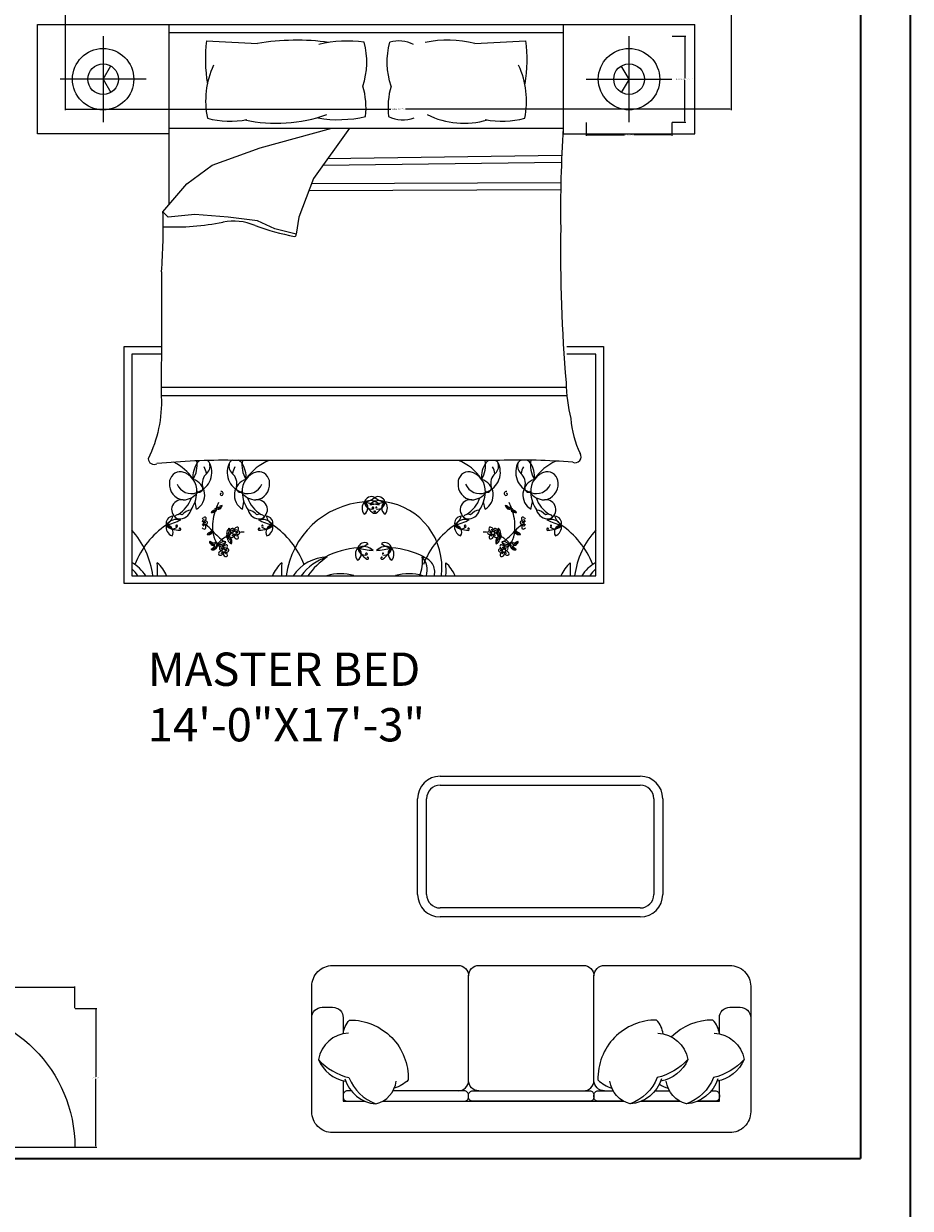
# Model space of a CAD drawing. Units: inches. Extents: x -10 to 502, y -868 to 56.
# Tile 13 of 14: x 298 to 458, y -264 to -50. Entities that reach past the tile are written whole.
import ezdxf

# ---------------------------------------------------------------- set-up
doc = ezdxf.new("R2010")
doc.units = ezdxf.units.IN
doc.header["$MEASUREMENT"] = 0
for name, color, linetype, lineweight in [('A-ANNO-DIMS', 2, 'Continuous', 18), ('A-AREA-IDEN', 7, 'Continuous', 18), ('A-DOOR', 4, 'Continuous', 25), ('A-FURN', 8, 'Continuous', 13), ('A-WALL', 7, 'Continuous', 35)]:
    doc.layers.add(name, color=color, linetype=linetype, lineweight=lineweight)
doc.styles.get("Standard").update_dxf_attribs({"font": 'arial.ttf'})
doc.dimstyles.get("Standard").update_dxf_attribs({"dimtxt": 0.18, "dimasz": 0.18, "dimexe": 0.18, "dimexo": 0.0625, "dimgap": 0.09, "dimtad": 0, "dimtih": 1, "dimtoh": 1, "dimdec": 0, "dimzin": 0, "dimdsep": 46, "dimlunit": 3, "dimtxsty": 'Standard', "dimcen": 0.09, "dimadec": 0, "dimazin": 0, "dimtfac": 1, "dimtdec": 0, "dimtofl": 0, "dimtmove": 0, "dimatfit": 3, "dimfxl": 1, "dimtolj": 1, "dimtzin": 0, "dimarcsym": 0})

# ---------------------------------------------------------------- blocks, each defined once
blk = doc.blocks.new('DOOR-SWING-25IN')
blk.add_line((25, 0), (0, 0))
blk.add_arc((25, 0), 25, 90, 180)
blk = doc.blocks.new('LAMP-BEDSIDE-LARGE')
for p, q in [((7.74, 0), (7.74, 15.47)), ((0, 7.74), (15.47, 7.74))]:
    blk.add_line(p, q)
for points in [[(7.74, 7.74), (6.35, 10.13)], [(7.74, 7.74), (6.35, 5.34)]]:
    blk.add_lwpolyline(points)
for radius in [5.53, 2.76]:
    blk.add_circle((7.74, 7.74), radius)
blk = doc.blocks.new('*D21')
at = {"layer": 'A-ANNO-DIMS', "color": 0, "lineweight": -2, "transparency": 16777216}
for p, q in [((305.7, -47.92), (305.7, -66.03)), ((425.7, -47.92), (425.7, -66.03)), ((305.88, -65.85), (364.4, -65.85)), ((425.52, -65.85), (367, -65.85))]:
    blk.add_line(p, q, dxfattribs=at)
at = {"layer": 'A-ANNO-DIMS', "color": 0, "transparency": 16777216}
for points in [[(305.88, -65.82), (305.88, -65.88), (305.7, -65.85)], [(425.52, -65.82), (425.52, -65.88), (425.7, -65.85)]]:
    blk.add_solid(points, dxfattribs=at)
at = {"layer": 'Defpoints', "color": 0, "transparency": 16777216}
for p in [(305.7, -47.85), (425.7, -47.85), (425.7, -65.85)]:
    blk.add_point(p, dxfattribs=at)
at = {"layer": 'A-ANNO-DIMS', "color": 0, "transparency": 16777216, "insert": (365.7, -65.85), "char_height": 0.18, "attachment_point": 5}
blk.add_mtext('\\A1;WINDOW 10\'-0" TYP.', dxfattribs=at)
blk = doc.blocks.new('*D25')
at = {"layer": 'A-ANNO-DIMS', "color": 0, "lineweight": -2, "transparency": 16777216}
for p, q in [((282.45, -227.79), (282.45, -223.92)), ((307.45, -227.79), (307.45, -223.92)), ((282.63, -224.1), (293.22, -224.1)), ((307.27, -224.1), (296.68, -224.1))]:
    blk.add_line(p, q, dxfattribs=at)
at = {"layer": 'A-ANNO-DIMS', "color": 0, "transparency": 16777216}
for points in [[(282.63, -224.07), (282.63, -224.13), (282.45, -224.1)], [(307.27, -224.07), (307.27, -224.13), (307.45, -224.1)]]:
    blk.add_solid(points, dxfattribs=at)
at = {"layer": 'Defpoints', "color": 0, "transparency": 16777216}
for p in [(282.45, -224.1), (282.45, -227.85), (307.45, -227.85)]:
    blk.add_point(p, dxfattribs=at)
at = {"layer": 'A-ANNO-DIMS', "color": 0, "transparency": 16777216, "insert": (294.95, -224.1), "char_height": 0.18, "attachment_point": 5}
blk.add_mtext('\\A1;BEDROOM DOOR 2\'-1" TYP.', dxfattribs=at)
blk = doc.blocks.new('*D26')
at = {"layer": 'A-ANNO-DIMS', "color": 0, "lineweight": -2, "transparency": 16777216}
for p, q in [((307.51, -227.85), (311.38, -227.85)), ((311.2, -228.03), (311.2, -240.17)), ((311.2, -252.67), (311.2, -240.53)), ((307.51, -252.85), (311.38, -252.85))]:
    blk.add_line(p, q, dxfattribs=at)
at = {"layer": 'A-ANNO-DIMS', "color": 0, "transparency": 16777216}
for points in [[(311.17, -228.03), (311.23, -228.03), (311.2, -227.85)], [(311.17, -252.67), (311.23, -252.67), (311.2, -252.85)]]:
    blk.add_solid(points, dxfattribs=at)
at = {"layer": 'Defpoints', "color": 0, "transparency": 16777216}
for p in [(307.45, -227.85), (311.2, -227.85), (307.45, -252.85)]:
    blk.add_point(p, dxfattribs=at)
at = {"layer": 'A-ANNO-DIMS', "color": 0, "transparency": 16777216, "insert": (311.2, -240.35), "char_height": 0.18, "attachment_point": 5}
blk.add_mtext('\\A1;2\'-1" TYP.', dxfattribs=at)
blk = doc.blocks.new('*D41')
at = {"layer": 'A-ANNO-DIMS', "color": 0, "lineweight": -2, "transparency": 16777216}
for p, q in [((415.08, -52.69), (417.52, -52.69)), ((417.34, -52.87), (417.34, -60.24)), ((417.34, -67.98), (417.34, -60.61)), ((415.08, -68.16), (417.52, -68.16))]:
    blk.add_line(p, q, dxfattribs=at)
at = {"layer": 'A-ANNO-DIMS', "color": 0, "transparency": 16777216}
for points in [[(417.31, -52.87), (417.37, -52.87), (417.34, -52.69)], [(417.31, -67.98), (417.37, -67.98), (417.34, -68.16)]]:
    blk.add_solid(points, dxfattribs=at)
at = {"layer": 'Defpoints', "color": 0, "transparency": 16777216}
for p in [(415.01, -52.69), (417.34, -52.69), (415.01, -68.16)]:
    blk.add_point(p, dxfattribs=at)
at = {"layer": 'A-ANNO-DIMS', "color": 0, "transparency": 16777216, "insert": (417.34, -60.43), "char_height": 0.18, "attachment_point": 5}
blk.add_mtext('\\A1;BEDSIDE LAMP 1\'-3 1/2" TYP.', dxfattribs=at)
blk = doc.blocks.new('*D42')
at = {"layer": 'A-ANNO-DIMS', "color": 0, "lineweight": -2, "transparency": 16777216}
for p, q in [((399.54, -68.22), (399.54, -70.66)), ((415.01, -68.22), (415.01, -70.66)), ((399.72, -70.48), (406.44, -70.48)), ((414.83, -70.48), (408.12, -70.48))]:
    blk.add_line(p, q, dxfattribs=at)
at = {"layer": 'A-ANNO-DIMS', "color": 0, "transparency": 16777216}
for points in [[(399.72, -70.45), (399.72, -70.51), (399.54, -70.48)], [(414.83, -70.45), (414.83, -70.51), (415.01, -70.48)]]:
    blk.add_solid(points, dxfattribs=at)
at = {"layer": 'Defpoints', "color": 0, "transparency": 16777216}
for p in [(399.54, -68.16), (415.01, -68.16), (415.01, -70.48)]:
    blk.add_point(p, dxfattribs=at)
at = {"layer": 'A-ANNO-DIMS', "color": 0, "transparency": 16777216, "insert": (407.28, -70.48), "char_height": 0.18, "attachment_point": 5}
blk.add_mtext('\\A1;1\'-3 1/2" TYP.', dxfattribs=at)

msp = doc.modelspace()

# ---------------------------------------------------------------- linework, layer by layer
at = {"layer": 'A-FURN'}
for p, q in [((300.7, -50.56), (419.12, -50.56)), ((324.38, -50.56), (324.38, -83.06)), ((395.44, -52.08), (324.38, -52.08)), ((324.38, -69.27), (395.44, -69.27)), ((340.83, -72.79), (353.75, -69.27)), ((356.92, -69.27), (350.43, -78.3)), ((332.2, -75.91), (340.83, -72.79)), ((395.12, -74.19), (352.96, -74.78)), ((327.64, -79.26), (332.2, -75.91)), ((395.07, -75.41), (352.07, -76.01)), ((350.43, -78.3), (347.79, -85.26)), ((323.32, -84.3), (327.64, -79.26)), ((395.02, -80.35), (349.58, -80.54)), ((395.01, -79.13), (350.04, -79.31)), ((324.28, -85.26), (323.32, -84.3)), ((329.08, -84.78), (324.28, -85.26)), ((335.08, -85.26), (329.08, -84.78)), ((340.35, -85.97), (335.08, -85.26)), ((347.79, -85.26), (347.31, -88.37)), ((343.47, -87.41), (340.35, -85.97)), ((347.31, -88.37), (343.47, -87.41)), ((316.33, -108.61), (323.03, -108.61)), ((316.33, -151.27), (316.33, -108.61)), ((396.1, -108.61), (402.66, -108.61)), ((402.66, -108.61), (402.66, -151.27)), ((323.03, -109.98), (317.7, -109.98)), ((317.7, -109.98), (317.7, -149.89)), ((401.29, -109.98), (396.07, -109.98)), ((401.29, -149.89), (401.29, -109.98)), ((395.97, -115.99), (323.02, -115.99)), ((396.09, -117.47), (323.02, -117.47)), ((383.95, -129.1), (335.87, -129.1)), ((329.37, -137.89), (329.11, -136.55)), ((337.65, -137.89), (337.91, -136.55)), ((381.34, -137.89), (381.08, -136.55)), ((389.62, -137.89), (389.88, -136.55)), ((402.66, -151.27), (316.33, -151.27)), ((317.7, -149.89), (401.29, -149.89)), ((373.25, -187.63), (409.31, -187.63)), ((370.82, -207.31), (370.82, -190.06)), ((411.73, -190.06), (411.73, -207.31)), ((409.31, -209.73), (373.25, -209.73))]:
    msp.add_line(p, q, dxfattribs=at)
at = {"layer": 'A-FURN', "ltscale": 0.03}
for p, q in [((373.25, -186.01), (409.31, -186.01)), ((369.2, -207.31), (369.2, -190.06)), ((413.35, -190.06), (413.35, -207.31)), ((409.31, -211.35), (373.25, -211.35))]:
    msp.add_line(p, q, dxfattribs=at)
at = {"layer": 'A-FURN'}
for points in [[(324.38, -70.29), (300.7, -70.29), (300.7, -50.56)], [(395.44, -50.56), (395.44, -70.29), (419.12, -70.29), (419.12, -50.56)], [(355.78, -240.87), (355.78, -244.57), (359.74, -244.57)], [(362.87, -244.57), (406.32, -244.57)], [(409.45, -244.57), (416.46, -244.57)]]:
    msp.add_lwpolyline(points, dxfattribs=at)
for points in [[(331.18, -53.51, 0.074897), (331.33, -61.24, -0.472817)], [(359.35, -61.68, 0.14099), (359.59, -53.79, 0.235245)], [(364.41, -61.68, -0.14099), (364.17, -53.79, -0.235245)], [(388.63, -53.51, -0.074897), (388.49, -61.24, 0.472817)], [(323.08, -95.14, 0.001242), (323.02, -117.61, -0.127202), (320.64, -128.81)], [(395.94, -115.06, 0.056112), (396.8, -121.58, 0.095341), (398.46, -127.85)], [(376.48, -242.69, 0.414214), (378.37, -240.81), (378.37, -221.98, 0.414214)], [(402.84, -242.69, -0.414214), (400.96, -240.81), (400.96, -221.98, -0.414214)], [(350.13, -229.51, -0.414214), (352.01, -227.63), (353.89, -227.63, -0.414214), (355.78, -229.51), (355.78, -232.43)], [(423.55, -232.43), (423.55, -229.51, -0.414214), (425.43, -227.63), (427.32, -227.63, -0.414214), (429.2, -229.51)], [(355.77, -232.43, -0.165541), (356.94, -229.94, -0.425989), (367.51, -240.73, -0.121523), (365, -242.21, 7.115464)], [(413.41, -232.43, 0.165541), (412.25, -229.94, 0.425989), (401.68, -240.73, 0.121523), (404.19, -242.21, -7.115464)], [(423.56, -232.43, 0.165541), (422.39, -229.94, 0.200231), (414.92, -232.97, 0.121523)], [(356.72, -232.31, 0.356772), (351.33, -237.06, 0.249542), (356.21, -240.97, -9.61688)], [(412.47, -232.31, -0.356772), (417.86, -237.06, -0.249542), (412.97, -240.97, 9.61688)], [(422.61, -232.31, -0.356772), (428, -237.06, -0.249542), (423.11, -240.97, 9.61688)], [(351.33, -237.06, 0.14773), (356.83, -240.3, 0.213343), (361.68, -245.04, 0.178662)], [(417.86, -237.06, -0.14773), (412.36, -240.3, -0.213343), (407.5, -245.04, -0.178662)], [(428, -237.06, -0.14773), (422.5, -240.3, -0.213343), (417.64, -245.04, -0.178662)], [(356.07, -240.55, 0.306663), (361.68, -245.04, 0.30633), (365.35, -240.94, -0.872847)], [(380.25, -242.69, -0.414214), (378.37, -240.81)], [(399.08, -242.69, 0.414214), (400.96, -240.81)], [(413.12, -240.55, -0.306663), (407.5, -245.04, -0.30633), (403.83, -240.94, 0.872847)], [(423.26, -240.55, -0.306663), (417.64, -245.04, -0.30633), (413.98, -240.94, 0.872847)], [(419.59, -244.57), (423.55, -244.57), (423.55, -240.87, -0.414214)], [(357.21, -242.69), (356.53, -242.69, 0.414214), (355.78, -243.44), (355.78, -243.82, 0.414214), (356.53, -244.57)], [(362.87, -244.57), (377.61, -244.57, 0.414214), (378.37, -243.82), (378.37, -243.44, 0.414214), (377.61, -242.69), (364.76, -242.69, 0.414214)], [(406.32, -244.57), (401.71, -244.57, -0.414214), (400.96, -243.82), (400.96, -243.44, -0.414214), (401.71, -242.69), (404.42, -242.69, -0.414214)], [(411.97, -242.69), (414.56, -242.69, -0.414214)], [(412.75, -241.48, 0.071865), (414.33, -242.21, -7.115464)], [(422.12, -242.69), (422.8, -242.69, -0.414214), (423.55, -243.44), (423.55, -243.82, -0.414214), (422.8, -244.57)], [(356.53, -244.57), (359.74, -244.57, 0.414214)], [(416.46, -244.57), (409.45, -244.57, -0.414214)], [(422.8, -244.57), (419.59, -244.57, -0.414214)]]:
    msp.add_lwpolyline(points, format="xyb", dxfattribs=at)
at = {"layer": 'A-FURN', "ltscale": 0.03}
msp.add_lwpolyline([(350.13, -223.86, -0.414214), (353.89, -220.1), (376.48, -220.1, -0.414214), (378.37, -221.98, -0.414214), (380.25, -220.1), (399.08, -220.1, -0.414214), (400.96, -221.98, -0.414214), (402.84, -220.1), (425.43, -220.1, -0.414214), (429.2, -223.86), (429.2, -246.46, -0.414214), (425.43, -250.22), (353.89, -250.22, -0.414214), (350.13, -246.46)], format="xyb", close=True, dxfattribs=at)
at = {"layer": 'A-FURN'}
msp.add_lwpolyline([(400.21, -244.57), (379.12, -244.57, -0.414214), (378.37, -243.82), (378.37, -243.44, -0.414214), (379.12, -242.69), (400.21, -242.69, -0.414214), (400.96, -243.44), (400.96, -243.82, -0.414214)], format="xyb", close=True, dxfattribs=at)
for centre in [(336.21, -142.18), (382.78, -142.18), (334.24, -145.36), (384.75, -145.36)]:
    msp.add_circle(centre, 0.302, dxfattribs=at)
for centre, radius, start, end in [((396.46, 1073.47), 1128.86, 266.68521, 267.14978), ((347.41, -96.36), 42.95, 82.2196, 99.497), ((356.48, -74.66), 21.1, 81.5249, 103.96), ((365.8, -59.41), 5.86, 63.3437, 106.1026), ((374.58, -74.23), 20.82, 76.3427, 101.1841), ((323.36, 1073.47), 1128.86, 272.85022, 273.31479), ((346.27, -64.35), 15.26, 155.1316, 191.7583), ((373.55, -64.35), 15.26, 348.2417, 24.8684), ((345.39, -65.63), 14.51, 354.0129, 15.8293), ((378.37, -65.63), 14.51, 164.1707, 185.9871), ((335.41, -52.12), 15.87, 255.1039, 281.0369), ((343.76, -40.84), 27.52, 258.0397, 289.2615), ((354.91, -46.85), 20.88, 259.8617, 283.6238), ((366.59, -61.46), 6.28, 245.0183, 288.5407), ((377.56, -53.29), 15.07, 243.8761, 286.1746), ((384.41, -52.12), 15.87, 258.9631, 284.8961), ((607.73, -83.74), 212.78, 176.1, 180.9282), ((214.74, -87.24), 108.62, 355.8294, 1.553), ((325.35, -42.36), 44.69, 267.4519, 281.3392), ((336.03, -95.63), 9.64, 66.2616, 101.3392), ((355.53, -43.62), 45.92, 250.1194, 259.3383), ((672.5, -91.48), 277.56, 179.1145, 184.8735), ((347.04, -88.47), 0.286, 268.8623, 19.7536), ((397.57, -128.45), 1.08, 246.5219, 33.8264), ((321.73, -128.73), 1.09, 183.98, 297.3412), ((334.46, -252.37), 123.28, 89.3433, 95.6887), ((321.27, -137.44), 8.96, 33.6671, 63.2997), ((333.28, -132.11), 4.57, 145.785, 184.7304), ((324.56, -129.98), 4.91, 328.8218, 9.1554), ((330.64, -130.41), 1.43, 120.0293, 142.325), ((328.36, -131.25), 3.77, 289.2822, 29.1751), ((330.03, -130.13), 1.77, 311.5653, 23.8354), ((330.64, -130.41), 1.43, 44.4517, 63.558), ((338.66, -131.25), 3.77, 150.8249, 250.7178), ((336.98, -130.13), 1.77, 156.1646, 228.4347), ((336.38, -130.41), 1.43, 113.229, 135.5483), ((336.38, -130.41), 1.43, 37.675, 66.7144), ((333.73, -132.11), 4.57, 355.2696, 34.215), ((342.46, -129.98), 4.91, 169.7133, 211.1782), ((345.75, -137.44), 8.96, 111.4941, 146.3329), ((373.25, -137.44), 8.96, 33.6671, 68.5059), ((385.26, -132.11), 4.57, 145.785, 184.7304), ((376.53, -129.98), 4.91, 328.8218, 10.2867), ((382.61, -130.41), 1.43, 113.2856, 142.325), ((380.33, -131.25), 3.77, 289.2822, 29.1751), ((382.61, -130.41), 1.43, 44.4517, 66.7144), ((382.01, -130.13), 1.77, 311.5653, 23.8354), ((387.58, -244.28), 115.23, 85.2402, 91.8035), ((390.63, -131.25), 3.77, 150.8249, 250.7178), ((388.96, -130.13), 1.77, 156.1646, 228.4347), ((388.36, -130.41), 1.43, 106.6343, 135.5483), ((388.36, -130.41), 1.43, 37.675, 72.5814), ((385.71, -132.11), 4.57, 355.2696, 34.215), ((394.43, -129.98), 4.91, 169.249, 211.1782), ((397.72, -137.44), 8.96, 113.6453, 146.3329), ((326.49, -133.14), 2, 84.4856, 181.0538), ((325.88, -134.62), 3.56, 355.2933, 76.921), ((332.82, -133.27), 2.43, 131.5653, 195.1471), ((327.79, -131.94), 3.4, 7.436, 29.9149), ((334.2, -133.27), 2.43, 344.8529, 48.4347), ((339.23, -131.94), 3.4, 150.0851, 172.564), ((341.14, -134.62), 3.56, 103.079, 184.7067), ((340.52, -133.14), 2, 358.9462, 95.5144), ((378.47, -133.14), 2, 84.4856, 181.0538), ((377.85, -134.62), 3.56, 355.2933, 76.921), ((384.79, -133.27), 2.43, 131.5653, 195.1471), ((379.76, -131.94), 3.4, 7.436, 29.9149), ((386.17, -133.27), 2.43, 344.8529, 48.4347), ((391.2, -131.94), 3.4, 150.0851, 172.564), ((393.11, -134.62), 3.56, 103.079, 184.7067), ((392.5, -133.14), 2, 358.9462, 95.5144), ((327.31, -133.42), 2.83, 174.9449, 262.8857), ((328.43, -132.35), 2.75, 201.5819, 291.4221), ((327.9, -135.34), 2.94, 299.9085, 73.1337), ((329.77, -134.1), 0.735, 257.3041, 15.1471), ((339.12, -135.34), 2.94, 106.8663, 240.0915), ((337.25, -134.1), 0.735, 164.8529, 282.6959), ((338.59, -132.35), 2.75, 248.5779, 338.4181), ((339.71, -133.42), 2.83, 277.1143, 5.0551), ((379.29, -133.42), 2.83, 174.9449, 262.8857), ((380.4, -132.35), 2.75, 201.5819, 291.4221), ((379.88, -135.34), 2.94, 299.9085, 73.1337), ((381.74, -134.1), 0.735, 257.3041, 15.1471), ((391.09, -135.34), 2.94, 106.8663, 240.0915), ((389.22, -134.1), 0.735, 164.8529, 282.6959), ((390.57, -132.35), 2.75, 248.5779, 338.4181), ((391.68, -133.42), 2.83, 277.1143, 5.0551), ((326.66, -137.98), 1.78, 80.264, 250.8688), ((323.14, -134.07), 5.59, 301.2614, 341.7045), ((326.82, -132.8), 3.44, 272.3591, 324.0401), ((323.09, -134.52), 6.35, 326.2883, 356.5076), ((333.28, -132.11), 4.57, 212.7011, 216.3445), ((333.85, -135.21), 0.228, 102.7051, 280.4384), ((333.82, -135.07), 0.371, 280.4384, 100.4136), ((333.73, -132.11), 4.57, 323.6555, 327.2989), ((340.2, -132.8), 3.44, 215.9599, 267.6409), ((343.93, -134.52), 6.35, 183.4924, 213.7117), ((343.88, -134.07), 5.59, 198.2955, 238.7386), ((340.36, -137.98), 1.78, 289.1312, 99.736), ((360.83, -151.98), 15.46, 94.4623, 172.255), ((360.9, -137.71), 1.71, 137.7873, 219.1145), ((358.95, -137.66), 1.29, 298.5391, 58.3627), ((360.86, -136.92), 1.28, 63.0274, 163.8037), ((359.56, -133.92), 2.64, 271.4585, 315.3727), ((360.63, -138.79), 2.44, 45.5411, 114.3101), ((362.86, -126.24), 10.82, 252.593, 267.2582), ((360.89, -136.61), 1.27, 177.7585, 283.852), ((363.33, -135.29), 3.91, 198.9159, 238.011), ((362.31, -138.79), 2.44, 65.6899, 134.4589), ((360.08, -126.24), 10.82, 272.7418, 287.407), ((362.08, -136.92), 1.28, 16.1963, 116.9726), ((363.38, -133.92), 2.64, 224.6273, 268.5415), ((359.61, -135.29), 3.91, 301.989, 341.0841), ((362.05, -136.61), 1.27, 256.148, 2.2415), ((363.99, -137.66), 1.29, 121.6373, 241.4609), ((362.04, -137.71), 1.71, 320.8855, 42.2127), ((361.61, -148.41), 11.97, 352.8636, 81.8197), ((378.64, -137.98), 1.78, 80.264, 250.8688), ((375.11, -134.07), 5.59, 301.2614, 341.7045), ((378.79, -132.8), 3.44, 272.3591, 324.0401), ((375.06, -134.52), 6.35, 326.2883, 356.5076), ((385.26, -132.11), 4.57, 212.7011, 216.3445), ((385.17, -135.07), 0.371, 79.5864, 259.5616), ((385.14, -135.21), 0.228, 259.5616, 77.2949), ((385.71, -132.11), 4.57, 323.6555, 327.2989), ((392.17, -132.8), 3.44, 215.9599, 267.6409), ((395.91, -134.52), 6.35, 183.4924, 213.7117), ((395.85, -134.07), 5.59, 198.2955, 238.7386), ((392.33, -137.98), 1.78, 289.1312, 99.736), ((326.24, -137.45), 2.22, 265.969, 344.3045), ((328.63, -140.4), 2.36, 96.1662, 141.5825), ((332.54, -138.74), 0.622, 101.3256, 154.4621), ((331.65, -136.63), 1.87, 280.2588, 300.656), ((332.08, -135.13), 3.34, 268.3264, 277.1302), ((342.06, -141.17), 9.81, 163.5842, 183.8277), ((331.24, -136.64), 1.9, 308.2101, 316.3071), ((332.41, -137.89), 0.568, 278.3432, 4.2869), ((332.1, -137.39), 0.992, 300.656, 332.6341), ((332.84, -138.04), 0.241, 55.7657, 157.4417), ((342.06, -141.17), 9.81, 153.0032, 159.8941), ((333.22, -137.82), 0.241, 84.3784, 186.0543), ((332.99, -136.85), 0.992, 269.1859, 301.164), ((333.28, -137.36), 0.568, 237.5332, 323.4768), ((332.73, -135.75), 1.9, 285.5129, 293.6099), ((333.97, -137.88), 0.622, 87.3579, 140.4944), ((332.54, -136.1), 1.87, 301.164, 321.5612), ((331.01, -135.77), 3.34, 324.6898, 333.4936), ((338.39, -140.4), 2.36, 38.4175, 83.8338), ((340.78, -137.45), 2.22, 195.6955, 274.031), ((361.15, -137.68), 0.167, 283.852, 219.9245), ((361.36, -138.45), 0.192, 238.011, 71.5592), ((361.39, -138.35), 0.0933, 71.5592, 188.0167), ((361.58, -138.45), 0.192, 108.4408, 301.989), ((361.55, -138.35), 0.0933, 351.9833, 108.4408), ((361.77, -137.61), 0.101, 320.1909, 256.0209), ((378.21, -137.45), 2.22, 265.969, 344.3045), ((380.6, -140.4), 2.36, 96.1662, 141.5825), ((386.46, -136.1), 1.87, 218.4388, 238.836), ((385.02, -137.88), 0.622, 39.5056, 92.6421), ((387.98, -135.77), 3.34, 206.5064, 215.3102), ((385.71, -137.36), 0.568, 216.5232, 302.4668), ((386, -136.85), 0.992, 238.836, 270.8141), ((386.26, -135.75), 1.9, 246.3901, 254.4871), ((376.93, -141.17), 9.81, 20.1059, 26.9968), ((385.78, -137.82), 0.241, 353.9457, 95.6216), ((386.58, -137.89), 0.568, 175.7131, 261.6568), ((386.15, -138.04), 0.241, 22.5583, 124.2343), ((386.9, -137.39), 0.992, 207.3659, 239.344), ((376.93, -141.17), 9.81, 356.1723, 16.4158), ((387.75, -136.64), 1.9, 223.6929, 231.7899), ((387.35, -136.63), 1.87, 239.344, 259.7412), ((386.91, -135.13), 3.34, 262.8698, 271.6736), ((386.45, -138.74), 0.622, 25.5379, 78.6744), ((392.76, -137.45), 2.22, 195.6955, 274.031), ((390.37, -140.4), 2.36, 38.4175, 83.8338), ((332.65, -153.51), 15.46, 124.3865, 158.5908), ((325.59, -141.11), 1.71, 167.7115, 249.0387), ((325.16, -140.44), 1.28, 92.9516, 193.728), ((322.54, -138.49), 2.64, 301.3827, 345.2969), ((325.9, -142.17), 2.44, 75.4653, 144.2343), ((321.57, -130.18), 10.82, 282.5173, 297.1824), ((323.87, -142.04), 1.29, 328.4633, 88.2869), ((326.49, -137.8), 3.91, 228.8402, 267.9352), ((325.03, -140.16), 1.27, 207.6827, 313.7762), ((326.3, -139.91), 1.09, 63.9755, 143.2681), ((325.79, -140.95), 0.167, 313.7762, 249.7183), ((330.78, -139.92), 0.503, 101.5637, 142.6358), ((330.37, -140.39), 0.302, 273.2768, 86.7232), ((330.72, -140.1), 0.288, 91.1081, 181.8675), ((331.31, -140.28), 0.916, 203.4276, 227.6104), ((331.02, -140.68), 0.623, 80.3487, 133.6538), ((330.91, -140.17), 0.493, 229.7889, 317.6792), ((330.38, -139.53), 0.725, 288.7263, 352.5032), ((330.36, -141.21), 0.701, 355.053, 68.3618), ((330.91, -141.33), 0.987, 83.0852, 105.7171), ((330.87, -139.56), 0.233, 345.2356, 144.9248), ((324.07, -149.52), 11.24, 43.1541, 52.0459), ((331.08, -140.32), 0.26, 317.6792, 80.3487), ((340.72, -139.91), 1.09, 36.7319, 116.0245), ((341.12, -142.17), 2.44, 35.7657, 104.5347), ((345.45, -130.18), 10.82, 242.8176, 257.4827), ((340.53, -137.8), 3.91, 272.0648, 311.1598), ((341.99, -140.16), 1.27, 226.2238, 332.3173), ((341.25, -140.89), 0.101, 290.2667, 226.2271), ((343.15, -142.04), 1.29, 91.7131, 211.5367), ((341.86, -140.44), 1.28, 346.272, 87.0484), ((344.48, -138.49), 2.64, 194.7031, 238.6173), ((341.43, -141.11), 1.71, 290.9613, 12.2885), ((334.37, -153.51), 15.46, 21.4092, 55.6135), ((384.62, -153.51), 15.46, 124.3865, 158.5908), ((377.13, -140.44), 1.28, 92.9516, 193.728), ((377.56, -141.11), 1.71, 167.7115, 249.0387), ((374.51, -138.49), 2.64, 301.3827, 345.2969), ((377.87, -142.17), 2.44, 75.4653, 144.2343), ((373.54, -130.18), 10.82, 282.5173, 297.1824), ((377.01, -140.16), 1.27, 207.6827, 313.7762), ((378.46, -137.8), 3.91, 228.8402, 267.9352), ((375.85, -142.04), 1.29, 328.4633, 88.2869), ((378.27, -139.91), 1.09, 63.9755, 143.2681), ((377.76, -140.95), 0.167, 313.7762, 249.7183), ((394.92, -149.52), 11.24, 127.9541, 136.8459), ((387.91, -140.32), 0.26, 99.6513, 222.3208), ((388.08, -140.17), 0.493, 222.3208, 310.2111), ((387.97, -140.68), 0.623, 46.3462, 99.6513), ((388.12, -139.56), 0.233, 35.0752, 194.7644), ((388.61, -139.53), 0.725, 187.4968, 251.2737), ((388.64, -141.21), 0.701, 111.6382, 184.947), ((388.09, -141.33), 0.987, 74.2829, 96.9148), ((388.27, -140.1), 0.288, 358.1325, 88.8919), ((387.68, -140.28), 0.916, 312.3896, 336.5724), ((388.21, -139.92), 0.503, 37.3642, 78.4363), ((388.63, -140.39), 0.302, 93.2768, 266.7232), ((392.7, -139.91), 1.09, 36.7319, 116.0245), ((393.1, -142.17), 2.44, 35.7657, 104.5347), ((397.43, -130.18), 10.82, 242.8176, 257.4827), ((392.51, -137.8), 3.91, 272.0648, 311.1598), ((393.96, -140.16), 1.27, 226.2238, 332.3173), ((393.22, -140.89), 0.101, 290.2667, 226.2271), ((395.12, -142.04), 1.29, 91.7131, 211.5367), ((396.46, -138.49), 2.64, 194.7031, 238.6173), ((393.84, -140.44), 1.28, 346.272, 87.0484), ((393.4, -141.11), 1.71, 290.9613, 12.2885), ((386.35, -153.51), 15.46, 21.4092, 55.6135), ((306.19, -151.98), 15.46, 7.745, 41.8856), ((326.33, -141.42), 0.0933, 101.4834, 217.9409), ((326.35, -141.52), 0.192, 267.9352, 101.4834), ((330.78, -140.95), 0.498, 217.7621, 259.0403), ((330.82, -141.25), 0.231, 232.4737, 355.053), ((331.84, -142.73), 0.622, 101.3256, 154.4621), ((330.94, -140.62), 1.87, 280.2588, 300.656), ((331.37, -139.12), 3.34, 268.3264, 277.1302), ((330.54, -140.62), 1.9, 308.2101, 316.3071), ((331.7, -141.87), 0.568, 278.3432, 4.2869), ((331.39, -141.37), 0.992, 300.656, 332.6341), ((332.14, -142.03), 0.241, 55.7657, 157.4417), ((337.17, -141.42), 4.92, 184.756, 209.2041), ((344.25, -130.95), 16.18, 222.2412, 232.1744), ((337.68, -147.95), 5.9, 120.544, 139.818), ((333.9, -141.73), 1.37, 304.5369, 16.3699), ((334.64, -142.04), 0.836, 272.8499, 356.1226), ((334.05, -142.36), 0.809, 321.7607, 7.9252), ((334.22, -143.52), 0.809, 8.7227, 54.8872), ((334.26, -144.17), 1.37, 0.278, 72.111), ((335.81, -142.12), 0.972, 127.3105, 187.9252), ((334.88, -143.67), 0.836, 20.5253, 88.5375), ((334.48, -142.01), 0.999, 355.0106, 41.658), ((335.58, -142.74), 0.299, 148.0499, 225.6268), ((337.68, -147.95), 5.9, 113.0501, 113.8477), ((336.13, -143.09), 0.951, 104.7558, 148.0499), ((335.6, -142.41), 0.595, 247.4086, 351.4386), ((335.88, -141.76), 0.411, 126.1046, 271.4281), ((335.83, -141.65), 0.295, 353.7526, 131.7054), ((335.77, -142.43), 0.2, 262.906, 7.132), ((335.56, -142), 0.415, 0.0645, 61.1507), ((335.65, -141.65), 0.474, 311.8413, 355.7877), ((336.63, -141.71), 0.503, 101.5637, 176.365), ((336.62, -142.74), 0.498, 151.2196, 259.0403), ((336.56, -141.89), 0.288, 91.1081, 181.8675), ((337.16, -142.07), 0.916, 203.4276, 227.6104), ((336.87, -142.47), 0.623, 80.3487, 133.6538), ((336.76, -141.96), 0.493, 229.7889, 317.6792), ((336.23, -141.32), 0.725, 288.7263, 352.5032), ((336.2, -143), 0.701, 355.053, 68.3618), ((336.75, -143.12), 0.987, 83.0852, 105.7171), ((336.72, -141.35), 0.233, 345.2356, 144.9248), ((336.93, -142.11), 0.26, 317.6792, 80.3487), ((337.68, -147.95), 5.9, 87.1071, 94.7585), ((340.67, -141.52), 0.192, 78.5166, 272.0648), ((340.69, -141.42), 0.0933, 322.0591, 78.5166), ((378.31, -141.42), 0.0933, 101.4834, 217.9409), ((378.33, -141.52), 0.192, 267.9352, 101.4834), ((381.32, -147.95), 5.9, 85.2415, 92.8929), ((382.06, -142.11), 0.26, 99.6513, 222.3208), ((382.23, -141.96), 0.493, 222.3208, 310.2111), ((382.12, -142.47), 0.623, 46.3462, 99.6513), ((382.27, -141.35), 0.233, 35.0752, 194.7644), ((382.77, -141.32), 0.725, 187.4968, 251.2737), ((382.79, -143), 0.701, 111.6382, 184.947), ((382.24, -143.12), 0.987, 74.2829, 96.9148), ((382.43, -141.89), 0.288, 358.1325, 88.8919), ((381.83, -142.07), 0.916, 312.3896, 336.5724), ((382.36, -141.71), 0.503, 3.635, 78.4363), ((382.37, -142.74), 0.498, 280.9597, 28.7804), ((383.39, -142.41), 0.595, 188.5614, 292.5914), ((383.16, -141.65), 0.295, 48.2946, 186.2474), ((383.34, -141.65), 0.474, 184.2123, 228.1587), ((383.44, -142), 0.415, 118.8493, 179.9355), ((383.23, -142.43), 0.2, 172.868, 277.094), ((383.11, -141.76), 0.411, 268.5719, 53.8954), ((382.86, -143.09), 0.951, 31.9501, 75.2442), ((384.12, -143.67), 0.836, 91.4625, 159.4747), ((384.73, -144.17), 1.37, 107.889, 179.722), ((384.52, -142.01), 0.999, 138.342, 184.9894), ((384.35, -142.04), 0.836, 183.8774, 267.1501), ((381.32, -147.95), 5.9, 66.1523, 66.9499), ((383.41, -142.74), 0.299, 314.3732, 31.9501), ((385.09, -141.73), 1.37, 163.6301, 235.4631), ((383.18, -142.12), 0.972, 352.0748, 52.6895), ((384.77, -143.52), 0.809, 125.1128, 171.2773), ((384.94, -142.36), 0.809, 172.0748, 218.2393), ((381.32, -147.95), 5.9, 40.182, 59.456), ((374.74, -130.95), 16.18, 307.8256, 317.7588), ((381.82, -141.42), 4.92, 330.7959, 355.244), ((386.86, -142.03), 0.241, 22.5583, 124.2343), ((387.29, -141.87), 0.568, 175.7131, 261.6568), ((387.6, -141.37), 0.992, 207.3659, 239.344), ((388.46, -140.62), 1.9, 223.6929, 231.7899), ((388.05, -140.62), 1.87, 239.344, 259.7412), ((387.62, -139.12), 3.34, 262.8698, 271.6736), ((387.16, -142.73), 0.622, 25.5379, 78.6744), ((388.17, -141.25), 0.231, 184.947, 307.5263), ((388.21, -140.95), 0.498, 280.9597, 322.2379), ((392.64, -141.52), 0.192, 78.5166, 272.0648), ((392.66, -141.42), 0.0933, 322.0591, 78.5166), ((412.8, -151.98), 15.46, 138.1144, 172.255), ((332.05, -143.82), 0.337, 146.8636, 236.9021), ((336.79, -136.4), 8.81, 235.1882, 238.8844), ((332.62, -143.33), 0.912, 199.4799, 267.6828), ((332.52, -143.67), 0.785, 212.8155, 277.3992), ((332.07, -144.2), 0.912, 266.9701, 338.2913), ((327.26, -137.69), 8.81, 302.6784, 306.3746), ((332.29, -144.92), 0.337, 214.3538, 304.3923), ((332.42, -143.64), 0.349, 238.8844, 314.2646), ((332.34, -144.42), 0.785, 280.3057, 17.1958), ((332.28, -144.51), 0.349, 306.3746, 21.7548), ((332.85, -144.28), 0.263, 19.3605, 201.7548), ((332.85, -144.08), 0.263, 311.8703, 134.2646), ((337.79, -146.48), 5.25, 153.7819, 158.2913), ((333.61, -142.89), 1.37, 247.2305, 319.0635), ((333.16, -143.35), 0.809, 264.4544, 310.6188), ((333.75, -143.67), 0.836, 218.3208, 298.8162), ((337.17, -141.42), 4.92, 214.0033, 222.4917), ((333.91, -144.94), 0.411, 126.1046, 271.4281), ((333.86, -144.83), 0.295, 353.7526, 131.7054), ((334.32, -144.7), 0.972, 70.0041, 130.6188), ((333.58, -145.18), 0.415, 0.0645, 61.1507), ((333.68, -144.82), 0.474, 311.8413, 355.7877), ((333.69, -143.52), 0.999, 297.7043, 344.3516), ((334.66, -144.89), 0.503, 101.5637, 176.365), ((334.59, -145.07), 0.288, 91.1081, 181.8675), ((334.9, -145.65), 0.623, 80.3487, 133.6538), ((334.25, -144.5), 0.725, 288.7263, 352.5032), ((334.75, -144.53), 0.233, 345.2356, 144.9248), ((334.96, -145.29), 0.26, 317.6792, 80.3487), ((335.98, -143.25), 0.972, 188.7227, 249.3375), ((334.73, -143.74), 0.999, 334.9899, 21.6373), ((336.67, -143.04), 0.231, 232.4737, 355.053), ((359.65, -160.26), 15.46, 94.4623, 117.4146), ((359.71, -146), 1.71, 137.7873, 219.1145), ((357.77, -145.94), 1.29, 298.5391, 58.3627), ((359.67, -145.2), 1.28, 63.0274, 163.8037), ((358.38, -142.2), 2.64, 271.4585, 315.3727), ((359.45, -147.07), 2.44, 45.5411, 114.3101), ((362.14, -143.58), 3.91, 198.9159, 238.011), ((361.68, -134.52), 10.82, 252.593, 267.2582), ((359.71, -144.89), 1.27, 177.7585, 283.852), ((363.49, -147.07), 2.44, 65.6899, 134.4589), ((361.26, -134.52), 10.82, 272.7418, 287.407), ((363.27, -145.2), 1.28, 16.1963, 116.9726), ((364.56, -142.2), 2.64, 224.6273, 268.5415), ((360.8, -143.58), 3.91, 301.989, 341.0841), ((363.23, -144.89), 1.27, 256.148, 2.2415), ((365.17, -145.94), 1.29, 121.6373, 241.4609), ((363.23, -146), 1.71, 320.8855, 42.2127), ((363.29, -160.26), 15.46, 62.5854, 85.5377), ((382.32, -143.04), 0.231, 184.947, 307.5263), ((384.26, -143.74), 0.999, 158.3627, 205.0101), ((383.01, -143.25), 0.972, 290.6625, 351.2773), ((384.03, -145.29), 0.26, 99.6513, 222.3208), ((384.09, -145.65), 0.623, 46.3462, 99.6513), ((384.25, -144.53), 0.233, 35.0752, 194.7644), ((384.74, -144.5), 0.725, 187.4968, 251.2737), ((384.67, -144.7), 0.972, 49.3812, 109.9959), ((385.38, -142.89), 1.37, 220.9365, 292.7695), ((385.3, -143.52), 0.999, 195.6484, 242.2957), ((384.4, -145.07), 0.288, 358.1325, 88.8919), ((384.33, -144.89), 0.503, 3.635, 78.4363), ((385.24, -143.67), 0.836, 241.1838, 321.6792), ((385.13, -144.83), 0.295, 48.2946, 186.2474), ((385.31, -144.82), 0.474, 184.2123, 228.1587), ((385.41, -145.18), 0.415, 118.8493, 179.9355), ((385.08, -144.94), 0.411, 268.5719, 53.8954), ((385.83, -143.35), 0.809, 229.3812, 275.5456), ((381.82, -141.42), 4.92, 317.5083, 325.9967), ((386.65, -144.42), 0.785, 162.8042, 259.6943), ((386.14, -144.08), 0.263, 45.7354, 228.1297), ((386.15, -144.28), 0.263, 338.2452, 160.6395), ((381.2, -146.48), 5.25, 21.7087, 26.2181), ((386.93, -144.2), 0.912, 201.7087, 273.0299), ((386.57, -143.64), 0.349, 225.7354, 301.1156), ((386.47, -143.67), 0.785, 262.6008, 327.1845), ((386.71, -144.51), 0.349, 158.2452, 233.6254), ((386.37, -143.33), 0.912, 272.3172, 340.5201), ((391.73, -137.69), 8.81, 233.6254, 237.3216), ((386.7, -144.92), 0.337, 235.6077, 325.6462), ((382.2, -136.4), 8.81, 301.1156, 304.8118), ((386.95, -143.82), 0.337, 303.0979, 33.1364), ((333.61, -145.92), 0.299, 148.0499, 225.6268), ((334.16, -146.27), 0.951, 104.7558, 148.0499), ((333.63, -145.59), 0.595, 247.4086, 351.4386), ((333.79, -145.61), 0.2, 262.906, 7.132), ((334.65, -145.92), 0.498, 151.2196, 259.0403), ((335.19, -145.25), 0.916, 203.4276, 227.6104), ((334.79, -145.14), 0.493, 229.7889, 317.6792), ((334.23, -146.18), 0.701, 355.053, 68.3618), ((334.78, -146.3), 0.987, 83.0852, 105.7171), ((334.7, -146.22), 0.231, 232.4737, 355.053), ((353.07, -154.05), 7.54, 91.272, 146.5383), ((355.78, -155.45), 9.39, 107.8504, 143.6964), ((360.72, -158.09), 13.97, 124.0123, 144.053), ((359.97, -145.96), 0.167, 283.852, 219.9245), ((360.17, -146.73), 0.192, 238.011, 71.5592), ((360.2, -146.64), 0.0933, 71.5592, 188.0167), ((362.77, -146.73), 0.192, 108.4408, 301.989), ((362.74, -146.64), 0.0933, 351.9833, 108.4408), ((362.95, -145.89), 0.101, 320.1909, 256.0209), ((363.16, -147.31), 6.92, 338.117, 6.6195), ((369.51, -149.24), 2.78, 346.3898, 79.0739), ((367.42, -148.86), 3.51, 342.8609, 41.9049), ((384.21, -145.14), 0.493, 222.3208, 310.2111), ((384.76, -146.18), 0.701, 111.6382, 184.947), ((384.29, -146.22), 0.231, 184.947, 307.5263), ((384.21, -146.3), 0.987, 74.2829, 96.9148), ((383.8, -145.25), 0.916, 312.3896, 336.5724), ((384.34, -145.92), 0.498, 280.9597, 28.7804), ((385.37, -145.59), 0.595, 188.5614, 292.5914), ((385.2, -145.61), 0.2, 172.868, 277.094), ((384.83, -146.27), 0.951, 31.9501, 75.2442), ((385.39, -145.92), 0.299, 314.3732, 31.9501), ((313.95, -154.05), 7.54, 33.4617, 60.1116), ((311.24, -155.45), 9.39, 36.3036, 46.4814), ((318.17, -152.31), 6.29, 22.5547, 48.9546), ((300.94, -148.93), 21.4, 357.4081, 3.6519), ((348.85, -152.31), 6.29, 131.0454, 157.4453), ((366.08, -148.93), 21.4, 176.3481, 182.5919), ((352.92, -148.93), 21.4, 357.4081, 3.6519), ((370.14, -152.31), 6.29, 22.5547, 48.9546), ((400.83, -152.31), 6.29, 131.0454, 157.4453), ((418.05, -148.93), 21.4, 176.3481, 182.5919), ((405.05, -154.05), 7.54, 119.8884, 146.5383), ((407.76, -155.45), 9.39, 133.5186, 143.6964), ((355.32, -158.02), 8.5, 73.5431, 107.0202), ((358.69, -162.41), 12.57, 94.3787, 95.6357), ((365.31, -171.02), 22.47, 109.7217, 109.9028), ((367.62, -158.02), 8.5, 72.9798, 106.4569), ((364.25, -162.41), 12.57, 84.3643, 85.6213), ((357.63, -171.02), 22.47, 70.0972, 70.2783), ((373.25, -190.06), 2.43, 90, 180), ((409.31, -190.06), 2.43, 0, 90), ((373.25, -207.31), 2.43, 180, 270), ((409.31, -207.31), 2.43, 270, 0)]:
    msp.add_arc(centre, radius, start, end, dxfattribs=at)
at = {"layer": 'A-FURN', "ltscale": 0.03}
for centre, start, end in [((373.25, -190.06), 90, 180), ((409.31, -190.06), 0, 90), ((373.25, -207.31), 180, 270), ((409.31, -207.31), 270, 0)]:
    msp.add_arc(centre, 4.05, start, end, dxfattribs=at)
at = {"layer": 'A-WALL'}
for p, q in [((457.95, 3.15), (457.95, -770.85)), ((448.95, -47.85), (448.95, -254.85)), ((282.45, -254.85), (448.95, -254.85))]:
    msp.add_line(p, q, dxfattribs=at)

# ---------------------------------------------------------------- block references
at = {"layer": 'A-DOOR', "extrusion": (0, 0, -1), "zscale": -1}
msp.add_blockref('DOOR-SWING-25IN', (-307.45, -252.85), dxfattribs=at)
at = {"layer": 'A-FURN', "rotation": 180}
msp.add_blockref('LAMP-BEDSIDE-LARGE', (320.28, -52.69), dxfattribs=at)
at = {"layer": 'A-FURN'}
msp.add_blockref('LAMP-BEDSIDE-LARGE', (399.54, -68.16), dxfattribs=at)

# ---------------------------------------------------------------- texts
at = {"layer": 'A-AREA-IDEN', "insert": (320.59, -163.73), "char_height": 6, "attachment_point": 1}
msp.add_mtext('MASTER BED\\P14\'-0"X17\'-3"', dxfattribs=at)

# ---------------------------------------------------------------- dimensions: what is measured, and where the dimension line sits
at = {"layer": 'A-ANNO-DIMS'}
for base, p1, p2, text, picture, middle in [((425.7, -65.85), (305.7, -47.85), (425.7, -47.85), 'WINDOW <> TYP.', '*D21', (365.7, -65.85)), ((415.01, -70.48), (399.54, -68.16), (415.01, -68.16), '<> TYP.', '*D42', (407.28, -70.48))]:
    dim = msp.add_linear_dim(base=base, p1=p1, p2=p2, text=text, dimstyle='Standard', override={"dimdec": 1, "dimlfac": 1, "dimrnd": 0, "dimzin": 1, "dimdsep": 46, "dimlunit": 4, "dimfrac": 2}, dxfattribs=at)
    dim.commit()
    dim.dimension.update_dxf_attribs({"geometry": picture, "text_midpoint": middle})
for base, p1, p2, angle, text, picture, middle in [((417.34, -52.69), (415.01, -68.16), (415.01, -52.69), 90, 'BEDSIDE LAMP <> TYP.', '*D41', (417.34, -60.43)), ((282.45, -224.1), (307.45, -227.85), (282.45, -227.85), 180, 'BEDROOM DOOR <> TYP.', '*D25', (294.95, -224.1)), ((311.2, -227.85), (307.45, -252.85), (307.45, -227.85), 90, '<> TYP.', '*D26', (311.2, -240.35))]:
    dim = msp.add_linear_dim(base=base, p1=p1, p2=p2, angle=angle, text=text, dimstyle='Standard', override={"dimdec": 1, "dimlfac": 1, "dimrnd": 0, "dimzin": 1, "dimdsep": 46, "dimlunit": 4, "dimfrac": 2}, dxfattribs=at)
    dim.commit()
    dim.dimension.update_dxf_attribs({"geometry": picture, "text_midpoint": middle})

doc.saveas('drawing.dxf')
